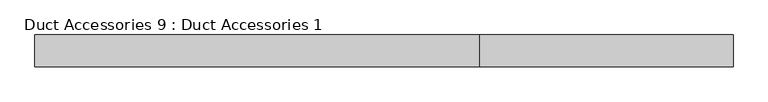
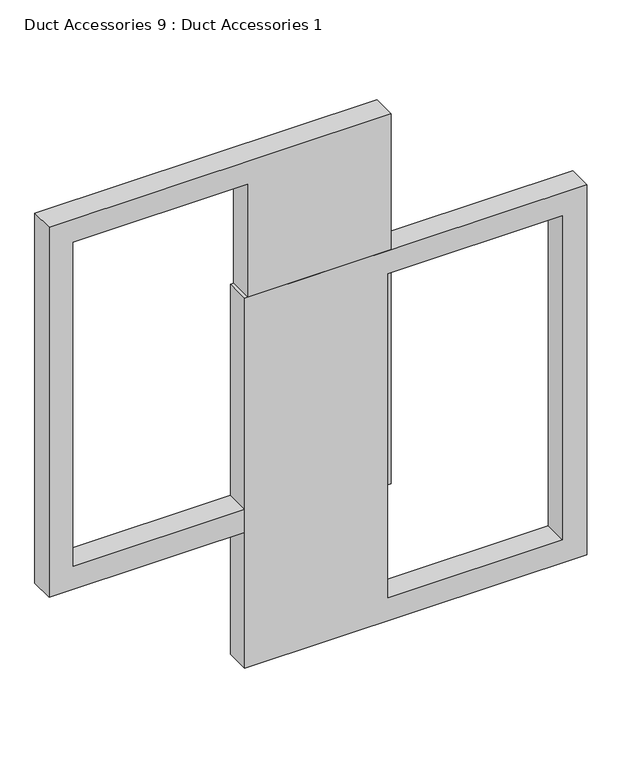
"""IFC4 building model written with IfcOpenShell, lengths in millimetres: damper geometry, Duct Accessories 9 : Duct Accessories 1."""

from ifc_helpers import new_model, si_unit, frame, origin, place, context, project, spatial, polyline, outline, extrude, source, transform, mapped, element, save


def duct_accessories_9_duct_accessories_1_ba76d1db(model_context):
    return source(origin(), model_context, "Body", "SweptSolid", [
        extrude(outline(polyline([(13991.1403114, -12928.36893), (12771.9403114, -12928.36893), (12771.9403114, -11861.56893), (13991.1403114, -11861.56893), (13991.1403114, -12928.36893)]), holes=[polyline([(13914.9403114, -12480.9324751), (13914.9403114, -11937.76893), (12848.1403114, -11937.76893), (12848.1403114, -12480.9324751), (13914.9403114, -12480.9324751)])]), frame((0.0, -447.4934478, 0.0), z_axis=(0.0, 1.0, 0.0), x_axis=(0.0, 0.0, 1.0)), (0.0, 0.0, 1.0), 76.2),
        extrude(outline(polyline([(14438.5767663, -12471.5606701), (14438.5767663, -13538.3606701), (13219.3767663, -13538.3606701), (13219.3767663, -12471.5606701), (14438.5767663, -12471.5606701)]), holes=[polyline([(14362.3767663, -12918.997125), (13295.5767663, -12918.997125), (13295.5767663, -13462.1606701), (14362.3767663, -13462.1606701), (14362.3767663, -12918.997125)])]), frame((0.0, -447.4934478, 0.0), z_axis=(0.0, 1.0, 0.0), x_axis=(0.0, 0.0, 1.0)), (0.0, 0.0, 1.0), 76.2),
    ])


if __name__ == "__main__":
    model = new_model("IFC4")
    model_context = context("Model", 3, world=origin())
    ifc_project = project(units=[si_unit("LENGTHUNIT", "METRE", prefix="MILLI")], contexts=[model_context])
    site = spatial("IfcSite", under=ifc_project)
    building = spatial("IfcBuilding", under=site)
    placement = place(None, origin())
    duct_accessories_9_duct_accessories_1_shape = duct_accessories_9_duct_accessories_1_ba76d1db(model_context)
    element("IfcDamper", 1, ObjectType="Duct Accessories 9 : Duct Accessories 1", at=placement, inside=building, context=model_context, shape_type="MappedRepresentation", body=[
        mapped(duct_accessories_9_duct_accessories_1_shape, transform((0.0, 0.0, 0.0), x_axis=(1.0, 0.0, 0.0), y_axis=(0.0, 1.0, 0.0), z_axis=(0.0, 0.0, 1.0))),
    ])
    save(model, "model.ifc")

# Revit data of these elements
# Element 1 (IfcDamper, "Duct Accessories 9 : Duct Accessories 1")
#   Materials on its faces: "border"
# Materials
#   "border": class "Generic", colour RGB 144 144 144, transparency 0, Cost = 0
